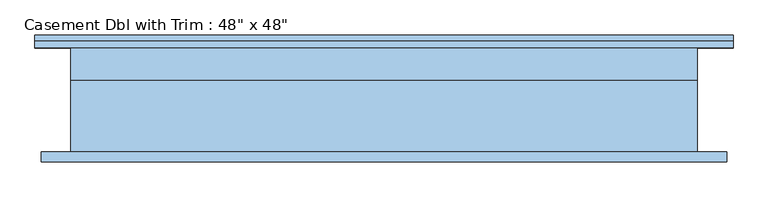
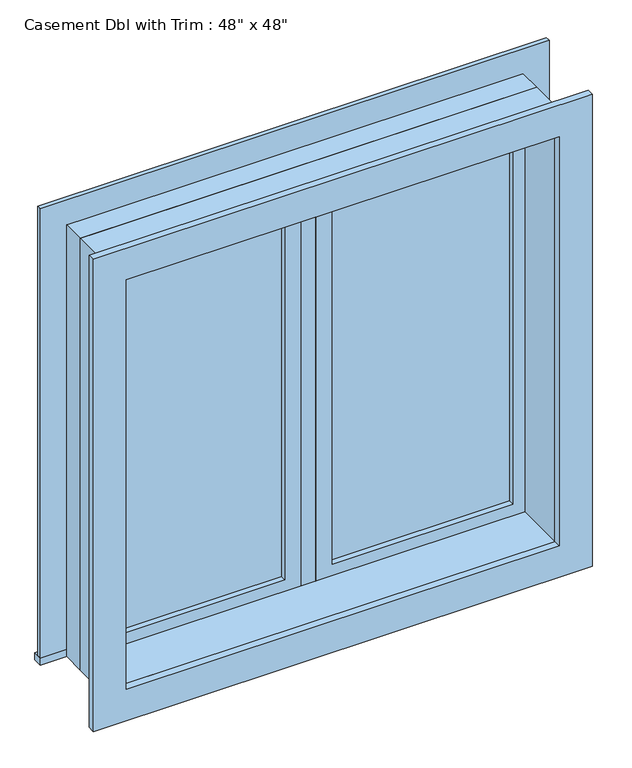
"""IFC4 building model written with IfcOpenShell, lengths in millimetres: window geometry."""

from ifc_helpers import new_model, si_unit, frame, origin, place, context, project, spatial, polyline, outline, extrude, source, transform, mapped, element, save


def window_0862ab64(model_context):
    return source(origin(), model_context, "Body", "SweptSolid", [
        extrude(outline(polyline([(63.5, 85.725), (546.1, 85.725), (546.1, 73.025), (63.5, 73.025), (63.5, 85.725)])), frame((0.0, 0.0, 977.9), z_axis=(0.0, 0.0, 1.0), x_axis=(1.0, 0.0, 0.0)), (0.0, 0.0, 1.0), 1092.2),
        extrude(outline(polyline([(2114.55, 19.05), (933.45, 19.05), (933.45, 590.55), (2114.55, 590.55), (2114.55, 19.05)]), holes=[polyline([(2070.1, 63.5), (2070.1, 546.1), (977.9, 546.1), (977.9, 63.5), (2070.1, 63.5)])]), frame((0.0, 57.15, 0.0), z_axis=(0.0, 1.0, 0.0), x_axis=(0.0, 0.0, 1.0)), (0.0, 0.0, 1.0), 44.45),
        extrude(outline(polyline([(19.05, 57.15), (-19.05, 57.15), (-19.05, 120.65), (19.05, 120.65), (19.05, 57.15)])), frame((0.0, 0.0, 933.45), z_axis=(0.0, 0.0, 1.0), x_axis=(1.0, 0.0, 0.0)), (0.0, 0.0, 1.0), 1181.1),
        extrude(outline(polyline([(-679.45, 146.05), (679.45, 146.05), (679.45, 120.65), (-679.45, 120.65), (-679.45, 146.05)])), frame((0.0, 0.0, 914.4), z_axis=(0.0, 0.0, 1.0), x_axis=(1.0, 0.0, 0.0)), (0.0, 0.0, 1.0), 19.05),
        extrude(outline(polyline([(2114.55, -590.55), (2114.55, 590.55), (933.45, 590.55), (933.45, 679.45), (2203.45, 679.45), (2203.45, -679.45), (933.45, -679.45), (933.45, -590.55), (2114.55, -590.55)])), frame((0.0, 120.65, 0.0), z_axis=(0.0, 1.0, 0.0), x_axis=(0.0, 0.0, 1.0)), (0.0, 0.0, 1.0), 12.7),
        extrude(outline(polyline([(2190.75, 666.75), (2190.75, -666.75), (857.25, -666.75), (857.25, 666.75), (2190.75, 666.75)]), holes=[polyline([(2101.85, 577.85), (946.15, 577.85), (946.15, -577.85), (2101.85, -577.85), (2101.85, 577.85)])]), frame((0.0, -101.6, 0.0), z_axis=(0.0, 1.0, 0.0), x_axis=(0.0, 0.0, 1.0)), (0.0, 0.0, 1.0), 19.05),
        extrude(outline(polyline([(-63.5, 73.025), (-546.1, 73.025), (-546.1, 85.725), (-63.5, 85.725), (-63.5, 73.025)])), frame((0.0, 0.0, 977.9), z_axis=(0.0, 0.0, 1.0), x_axis=(1.0, 0.0, 0.0)), (0.0, 0.0, 1.0), 1092.2),
        extrude(outline(polyline([(2114.55, -590.55), (933.45, -590.55), (933.45, -19.05), (2114.55, -19.05), (2114.55, -590.55)]), holes=[polyline([(2070.1, -546.1), (2070.1, -63.5), (977.9, -63.5), (977.9, -546.1), (2070.1, -546.1)])]), frame((0.0, 57.15, 0.0), z_axis=(0.0, 1.0, 0.0), x_axis=(0.0, 0.0, 1.0)), (0.0, 0.0, 1.0), 44.45),
        extrude(outline(polyline([(2133.6, -609.6), (914.4, -609.6), (914.4, 609.6), (2133.6, 609.6), (2133.6, -609.6)]), holes=[polyline([(2101.85, -577.85), (2101.85, 577.85), (946.15, 577.85), (946.15, -577.85), (2101.85, -577.85)])]), frame((0.0, -82.55, 0.0), z_axis=(0.0, 1.0, 0.0), x_axis=(0.0, 0.0, 1.0)), (0.0, 0.0, 1.0), 139.7),
        extrude(outline(polyline([(2133.6, 609.6), (2133.6, -609.6), (914.4, -609.6), (914.4, 609.6), (2133.6, 609.6)]), holes=[polyline([(2114.55, 590.55), (933.45, 590.55), (933.45, -590.55), (2114.55, -590.55), (2114.55, 590.55)])]), frame((0.0, 57.15, 0.0), z_axis=(0.0, 1.0, 0.0), x_axis=(0.0, 0.0, 1.0)), (0.0, 0.0, 1.0), 63.5),
    ])


if __name__ == "__main__":
    model = new_model("IFC4")
    model_context = context("Model", 3, world=origin())
    ifc_project = project(units=[si_unit("LENGTHUNIT", "METRE", prefix="MILLI")], contexts=[model_context])
    site = spatial("IfcSite", under=ifc_project)
    building = spatial("IfcBuilding", under=site)
    placement = place(None, origin())
    window_shape = window_0862ab64(model_context)
    element("IfcWindow", 1, ObjectType="Casement Dbl with Trim : 48\" x 48\"", at=placement, inside=building, context=model_context, shape_type="MappedRepresentation", body=[
        mapped(window_shape, transform((0.0, 0.0, 0.0), x_axis=(1.0, 0.0, 0.0), y_axis=(0.0, 1.0, 0.0), z_axis=(0.0, 0.0, 1.0))),
    ])
    save(model, "model.ifc")

# Revit data of these elements
# Type "Casement Dbl with Trim : 48\" x 48\""
#   Type Mark = "17"
#   Construction Type Id = "GSP4R"
#   Assembly Code = "B2020100"
#   Analytic Construction = "1/8 in Pilkington single glazing"
#   Visual Light Transmittance = 0.9
#   Solar Heat Gain Coefficient = 0.78
#   Heat Transfer Coefficient (U) = 0.6496 BTU/(h·ft²·°F)
#   Height = 4' - 0"
#   Default Sill Height = 3' - 0"
#   Trim Projection - Ext. = 0' - 0 1/2"
#   Trim Projection - Int. = 0' - 0 3/4"
#   Trim Width - Exterior = 0' - 3 1/2"
#   Trim Width - Interior = 0' - 3 1/2"
#   Width = 4' - 0"
#   Window Inset = 0' - 0 3/4"
#   Define Thermal Properties by = 1
#   Glass Pane Material = Glass
#   Sash Material = Sash
#   Trim Exterior Material = Trim
#   Trim Interior Material = Trim
#   Wall Closure = (empty or 0)
# Element 1 (IfcWindow, "Casement Dbl with Trim : 48\" x 48\"")
#   Materials on its faces: "Sash", "Trim", "Glass"
# Materials
#   "Glass": class "Glass", colour RGB 0 128 192, transparency 0.75, Description = "Soda Lime Glass", Cost = 0
#   "Sash": class "Wood", colour RGB 224 178 126, transparency 0
#   "Trim": class "Wood", colour RGB 224 178 126, transparency 0
